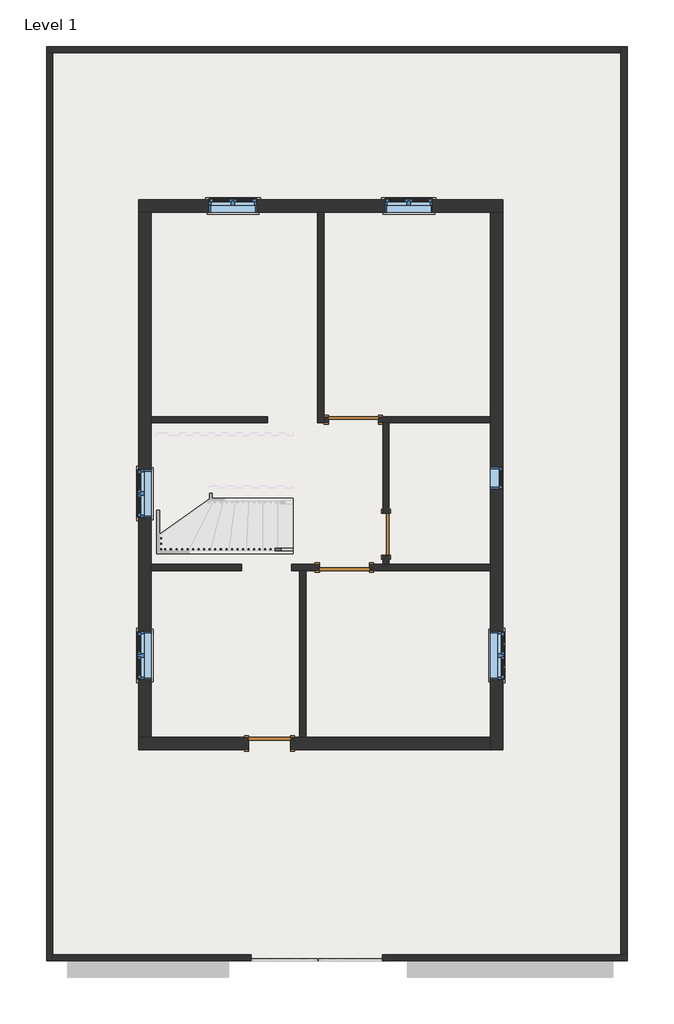
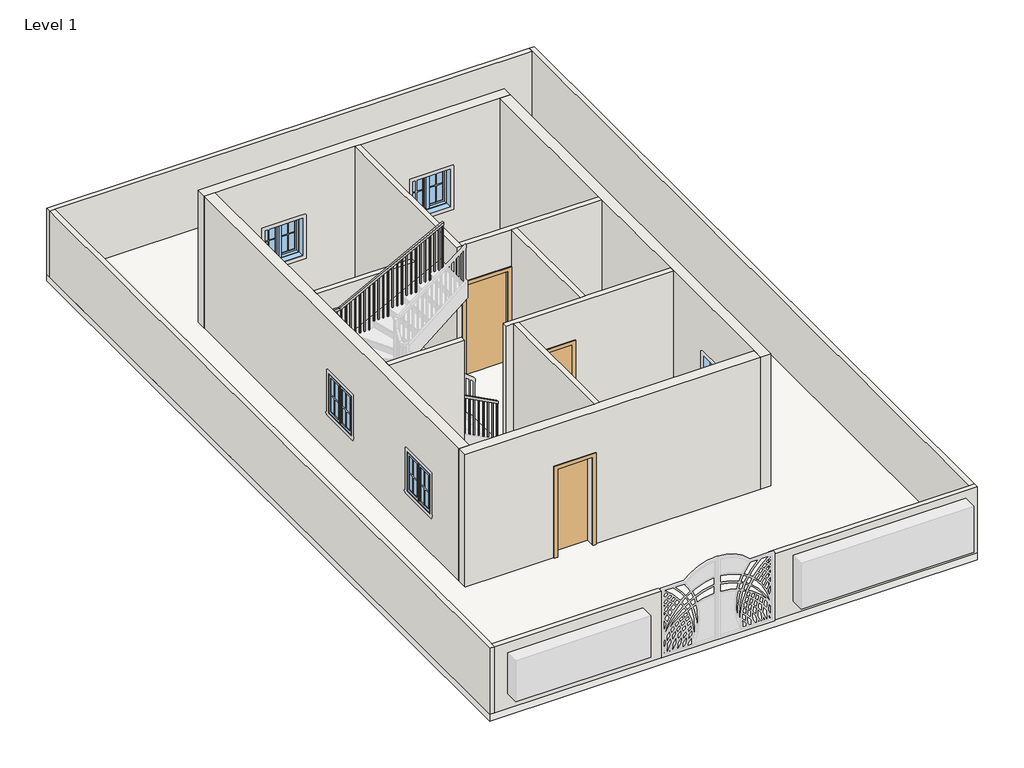
# One storey, part 1 of 2: 16 walls, 6 windows, 4 doors, 1 railing, 1 slab.
"""IFC4 building model written with IfcOpenShell, lengths in millimetres."""

from ifc_helpers import new_model, si_unit, frame, origin, origin_with_axes, place, context, project, spatial, polyline, outline, extrude, faceted_brep, transform, mapped, element, save
from components import door_d8f5dbb5, door_85036156, door_305aa2a5, door_e5f9f3c4, window_aa618e30, window_339605e1

model = new_model("IFC4")

# Units and contexts
model_context = context("Model", 3, world=origin())
ifc_project = project(units=[si_unit("LENGTHUNIT", "METRE", prefix="MILLI")], contexts=[model_context])

# Site, building, storey
site = spatial("IfcSite", under=ifc_project)
building = spatial("IfcBuilding", under=site)
storey = spatial("IfcBuildingStorey", under=building, Name="Level 1", Elevation=0.0)

# Doors
placement = place(None, origin())
door_shape = door_d8f5dbb5(model_context)
element("IfcDoor", 1, ObjectType="Single-Flush : 30\" x 80\"", at=placement, inside=storey, context=model_context, shape_type="MappedRepresentation", body=[
    mapped(door_shape, transform((-82.2715692, -955.3070853, 0.0), x_axis=(0.0, -1.0, 0.0), y_axis=(1.0, 0.0, 0.0), z_axis=(0.0, 0.0, 1.0))),
])
door_2_shape = door_85036156(model_context)
element("IfcDoor", 2, ObjectType="Single-Flush : 30\" x 80\"", at=placement, inside=storey, context=model_context, shape_type="MappedRepresentation", body=[
    mapped(door_2_shape, transform((-2212.5949167, -4784.3570853, 0.0), x_axis=(-1.0, 0.0, 0.0), y_axis=(0.0, -1.0, 0.0), z_axis=(0.0, 0.0, 1.0))),
])
door_3_shape = door_305aa2a5(model_context)
element("IfcDoor", 3, ObjectType="Single-Flush : 36\" x 84\"", at=placement, inside=storey, context=model_context, shape_type="MappedRepresentation", body=[
    mapped(door_3_shape, transform((-677.5332429, 1140.1929147, 0.0), x_axis=(-1.0, 0.0, 0.0), y_axis=(0.0, -1.0, 0.0), z_axis=(0.0, 0.0, 1.0))),
])
door_4_shape = door_e5f9f3c4(model_context)
element("IfcDoor", 4, ObjectType="Single-Flush : 36\" x 84\"", at=placement, inside=storey, context=model_context, shape_type="MappedRepresentation", body=[
    mapped(door_4_shape, transform((-842.6332429, -1564.9070853, 0.0), x_axis=(-1.0, 0.0, 0.0), y_axis=(0.0, -1.0, 0.0), z_axis=(0.0, 0.0, 1.0))),
])

# Railing
element("IfcRailing", 5, ObjectType="Handrail - Rectangular", at=placement, inside=storey, context=model_context, shape_type="SolidModel", body=[
    faceted_brep([(-1783.4132248, -1260.1070853, 1083.7333333), (-1783.4132248, -1260.1070853, 1026.2742652), (-1783.4132248, -1209.3070853, 1026.2742652), (-1783.4132248, -1209.3070853, 1083.7333333), (-4041.1382869, -1260.1070853, 2277.0239201), (-4053.7373514, -1260.1070853, 2226.2239201), (-4053.7373514, -1209.3070853, 2226.2239201), (-4041.1382869, -1209.3070853, 2277.0239201), (-4225.5449167, -1260.1070853, 2277.0239201), (-4225.5449167, -1260.1070853, 2226.2239201), (-4174.7449167, -1209.3070853, 2226.2239201), (-4174.7449167, -1209.3070853, 2277.0239201), (-4225.5449167, -972.7952032, 2277.0239201), (-4225.5449167, -964.8446271, 2226.2239201), (-4174.7449167, -964.8446271, 2226.2239201), (-4174.7449167, -972.7952032, 2277.0239201), (-4225.5449167, 560.7810325, 2769.1094132), (-4225.5449167, 568.7316087, 2718.3094132), (-4174.7449167, 568.7316087, 2718.3094132), (-4174.7449167, 560.7810325, 2769.1094132), (-4225.5449167, 848.0929147, 2769.1094132), (-4225.5449167, 848.0929147, 2718.3094132), (-4174.7449167, 797.2929147, 2718.3094132), (-4174.7449167, 797.2929147, 2769.1094132), (-4041.1382869, 848.0929147, 2769.1094132), (-4028.5392223, 848.0929147, 2718.3094132), (-4028.5392223, 797.2929147, 2718.3094132), (-4041.1382869, 797.2929147, 2769.1094132), (-1783.4132248, 848.0929147, 3962.4), (-1783.4132248, 797.2929147, 3962.4), (-1783.4132248, 797.2929147, 3904.9409318), (-1783.4132248, 848.0929147, 3904.9409318)], [[[0, 1, 2, 3]], [[1, 0, 4, 5]], [[2, 1, 5, 6]], [[3, 2, 6, 7]], [[0, 3, 7, 4]], [[5, 4, 8, 9]], [[6, 5, 9, 10]], [[7, 6, 10, 11]], [[4, 7, 11, 8]], [[9, 8, 12, 13]], [[10, 9, 13, 14]], [[11, 10, 14, 15]], [[8, 11, 15, 12]], [[13, 12, 16, 17]], [[14, 13, 17, 18]], [[15, 14, 18, 19]], [[12, 15, 19, 16]], [[17, 16, 20, 21]], [[18, 17, 21, 22]], [[19, 18, 22, 23]], [[16, 19, 23, 20]], [[21, 20, 24, 25]], [[22, 21, 25, 26]], [[23, 22, 26, 27]], [[20, 23, 27, 24]], [[28, 29, 30, 31]], [[25, 24, 28, 31]], [[26, 25, 31, 30]], [[27, 26, 30, 29]], [[24, 27, 29, 28]]]),
    extrude(outline(polyline([(3857.6597858, -1872.8699167), (2878.6666667, -1872.8699167), (2878.6666667, -1853.8199167), (3867.7284102, -1853.8199167), (3857.6597858, -1872.8699167)])), frame((0.0, 813.1679147, 0.0), z_axis=(0.0, 1.0, 0.0), x_axis=(0.0, 0.0, 1.0)), (0.0, 0.0, 1.0), 19.05),
    extrude(outline(polyline([(3803.9604556, -1974.4699167), (2878.6666667, -1974.4699167), (2878.6666667, -1955.4199167), (3814.02908, -1955.4199167), (3803.9604556, -1974.4699167)])), frame((0.0, 813.1679147, 0.0), z_axis=(0.0, 1.0, 0.0), x_axis=(0.0, 0.0, 1.0)), (0.0, 0.0, 1.0), 19.05),
    extrude(outline(polyline([(3750.2611254, -2076.0699167), (2709.3333333, -2076.0699167), (2709.3333333, -2057.0199167), (3760.3297498, -2057.0199167), (3750.2611254, -2076.0699167)])), frame((0.0, 813.1679147, 0.0), z_axis=(0.0, 1.0, 0.0), x_axis=(0.0, 0.0, 1.0)), (0.0, 0.0, 1.0), 19.05),
    extrude(outline(polyline([(3696.5617952, -2177.6699167), (2709.3333333, -2177.6699167), (2709.3333333, -2158.6199167), (3706.6304196, -2158.6199167), (3696.5617952, -2177.6699167)])), frame((0.0, 813.1679147, 0.0), z_axis=(0.0, 1.0, 0.0), x_axis=(0.0, 0.0, 1.0)), (0.0, 0.0, 1.0), 19.05),
    extrude(outline(polyline([(3642.862465, -2279.2699167), (2709.3333333, -2279.2699167), (2709.3333333, -2260.2199167), (3652.9310894, -2260.2199167), (3642.862465, -2279.2699167)])), frame((0.0, 813.1679147, 0.0), z_axis=(0.0, 1.0, 0.0), x_axis=(0.0, 0.0, 1.0)), (0.0, 0.0, 1.0), 19.05),
    extrude(outline(polyline([(3589.1631348, -2380.8699167), (2540.0, -2380.8699167), (2540.0, -2361.8199167), (3599.2317592, -2361.8199167), (3589.1631348, -2380.8699167)])), frame((0.0, 813.1679147, 0.0), z_axis=(0.0, 1.0, 0.0), x_axis=(0.0, 0.0, 1.0)), (0.0, 0.0, 1.0), 19.05),
    extrude(outline(polyline([(3535.4638046, -2482.4699167), (2540.0, -2482.4699167), (2540.0, -2463.4199167), (3545.532429, -2463.4199167), (3535.4638046, -2482.4699167)])), frame((0.0, 813.1679147, 0.0), z_axis=(0.0, 1.0, 0.0), x_axis=(0.0, 0.0, 1.0)), (0.0, 0.0, 1.0), 19.05),
    extrude(outline(polyline([(3481.7644744, -2584.0699167), (2540.0, -2584.0699167), (2540.0, -2565.0199167), (3491.8330988, -2565.0199167), (3481.7644744, -2584.0699167)])), frame((0.0, 813.1679147, 0.0), z_axis=(0.0, 1.0, 0.0), x_axis=(0.0, 0.0, 1.0)), (0.0, 0.0, 1.0), 19.05),
    extrude(outline(polyline([(3428.0651442, -2685.6699167), (2370.6666667, -2685.6699167), (2370.6666667, -2666.6199167), (3438.1337686, -2666.6199167), (3428.0651442, -2685.6699167)])), frame((0.0, 813.1679147, 0.0), z_axis=(0.0, 1.0, 0.0), x_axis=(0.0, 0.0, 1.0)), (0.0, 0.0, 1.0), 19.05),
    extrude(outline(polyline([(3374.365814, -2787.2699167), (2370.6666667, -2787.2699167), (2370.6666667, -2768.2199167), (3384.4344384, -2768.2199167), (3374.365814, -2787.2699167)])), frame((0.0, 813.1679147, 0.0), z_axis=(0.0, 1.0, 0.0), x_axis=(0.0, 0.0, 1.0)), (0.0, 0.0, 1.0), 19.05),
    extrude(outline(polyline([(3320.6664838, -2888.8699167), (2370.6666667, -2888.8699167), (2370.6666667, -2869.8199167), (3330.7351082, -2869.8199167), (3320.6664838, -2888.8699167)])), frame((0.0, 813.1679147, 0.0), z_axis=(0.0, 1.0, 0.0), x_axis=(0.0, 0.0, 1.0)), (0.0, 0.0, 1.0), 19.05),
    extrude(outline(polyline([(3266.9671536, -2990.4699167), (2201.3333333, -2990.4699167), (2201.3333333, -2971.4199167), (3277.035778, -2971.4199167), (3266.9671536, -2990.4699167)])), frame((0.0, 813.1679147, 0.0), z_axis=(0.0, 1.0, 0.0), x_axis=(0.0, 0.0, 1.0)), (0.0, 0.0, 1.0), 19.05),
    extrude(outline(polyline([(3213.2678234, -3092.0699167), (2201.3333333, -3092.0699167), (2201.3333333, -3073.0199167), (3223.3364478, -3073.0199167), (3213.2678234, -3092.0699167)])), frame((0.0, 813.1679147, 0.0), z_axis=(0.0, 1.0, 0.0), x_axis=(0.0, 0.0, 1.0)), (0.0, 0.0, 1.0), 19.05),
    extrude(outline(polyline([(3159.5684932, -3193.6699167), (2201.3333333, -3193.6699167), (2201.3333333, -3174.6199167), (3169.6371176, -3174.6199167), (3159.5684932, -3193.6699167)])), frame((0.0, 813.1679147, 0.0), z_axis=(0.0, 1.0, 0.0), x_axis=(0.0, 0.0, 1.0)), (0.0, 0.0, 1.0), 19.05),
    extrude(outline(polyline([(3105.869163, -3295.2699167), (2201.3333333, -3295.2699167), (2201.3333333, -3276.2199167), (3115.9377874, -3276.2199167), (3105.869163, -3295.2699167)])), frame((0.0, 813.1679147, 0.0), z_axis=(0.0, 1.0, 0.0), x_axis=(0.0, 0.0, 1.0)), (0.0, 0.0, 1.0), 19.05),
    extrude(outline(polyline([(3052.1698328, -3396.8699167), (2032.0, -3396.8699167), (2032.0, -3377.8199167), (3062.2384572, -3377.8199167), (3052.1698328, -3396.8699167)])), frame((0.0, 813.1679147, 0.0), z_axis=(0.0, 1.0, 0.0), x_axis=(0.0, 0.0, 1.0)), (0.0, 0.0, 1.0), 19.05),
    extrude(outline(polyline([(2998.4705026, -3498.4699167), (2032.0, -3498.4699167), (2032.0, -3479.4199167), (3008.539127, -3479.4199167), (2998.4705026, -3498.4699167)])), frame((0.0, 813.1679147, 0.0), z_axis=(0.0, 1.0, 0.0), x_axis=(0.0, 0.0, 1.0)), (0.0, 0.0, 1.0), 19.05),
    extrude(outline(polyline([(2944.7711724, -3600.0699167), (2032.0, -3600.0699167), (2032.0, -3581.0199167), (2954.8397968, -3581.0199167), (2944.7711724, -3600.0699167)])), frame((0.0, 813.1679147, 0.0), z_axis=(0.0, 1.0, 0.0), x_axis=(0.0, 0.0, 1.0)), (0.0, 0.0, 1.0), 19.05),
    extrude(outline(polyline([(2891.0718422, -3701.6699167), (2032.0, -3701.6699167), (2032.0, -3682.6199167), (2901.1404666, -3682.6199167), (2891.0718422, -3701.6699167)])), frame((0.0, 813.1679147, 0.0), z_axis=(0.0, 1.0, 0.0), x_axis=(0.0, 0.0, 1.0)), (0.0, 0.0, 1.0), 19.05),
    extrude(outline(polyline([(2837.372512, -3803.2699167), (1862.6666667, -3803.2699167), (1862.6666667, -3784.2199167), (2847.4411364, -3784.2199167), (2837.372512, -3803.2699167)])), frame((0.0, 813.1679147, 0.0), z_axis=(0.0, 1.0, 0.0), x_axis=(0.0, 0.0, 1.0)), (0.0, 0.0, 1.0), 19.05),
    extrude(outline(polyline([(2783.6731818, -3904.8699167), (1862.6666667, -3904.8699167), (1862.6666667, -3885.8199167), (2793.7418062, -3885.8199167), (2783.6731818, -3904.8699167)])), frame((0.0, 813.1679147, 0.0), z_axis=(0.0, 1.0, 0.0), x_axis=(0.0, 0.0, 1.0)), (0.0, 0.0, 1.0), 19.05),
    extrude(outline(polyline([(2729.9738516, -4006.4699167), (1862.6666667, -4006.4699167), (1862.6666667, -3987.4199167), (2740.042476, -3987.4199167), (2729.9738516, -4006.4699167)])), frame((0.0, 813.1679147, 0.0), z_axis=(0.0, 1.0, 0.0), x_axis=(0.0, 0.0, 1.0)), (0.0, 0.0, 1.0), 19.05),
    extrude(outline(polyline([(-4108.0699167, 832.2179147), (-4089.0199167, 832.2179147), (-4089.0199167, 813.1679147), (-4108.0699167, 813.1679147), (-4108.0699167, 832.2179147)])), frame((0.0, 0.0, 1862.6666667), z_axis=(0.0, 0.0, 1.0), x_axis=(1.0, 0.0, 0.0)), (0.0, 0.0, 1.0), 855.6427466),
    extrude(outline(polyline([(-4209.6699167, 787.7679147), (-4209.6699167, 806.8179147), (-4190.6199167, 806.8179147), (-4190.6199167, 787.7679147), (-4209.6699167, 787.7679147)])), frame((0.0, 0.0, 1862.6666667), z_axis=(0.0, 0.0, 1.0), x_axis=(1.0, 0.0, 0.0)), (0.0, 0.0, 1.0), 855.6427466),
    extrude(outline(polyline([(-4209.6699167, 686.1679147), (-4209.6699167, 705.2179147), (-4190.6199167, 705.2179147), (-4190.6199167, 686.1679147), (-4209.6699167, 686.1679147)])), frame((0.0, 0.0, 1862.6666667), z_axis=(0.0, 0.0, 1.0), x_axis=(1.0, 0.0, 0.0)), (0.0, 0.0, 1.0), 855.6427466),
    extrude(outline(polyline([(-4209.6699167, 584.5679147), (-4209.6699167, 603.6179147), (-4190.6199167, 603.6179147), (-4190.6199167, 584.5679147), (-4209.6699167, 584.5679147)])), frame((0.0, 0.0, 1862.6666667), z_axis=(0.0, 0.0, 1.0), x_axis=(1.0, 0.0, 0.0)), (0.0, 0.0, 1.0), 855.6427466),
    extrude(outline(polyline([(502.0179147, 2696.9026907), (502.0179147, 1693.3333333), (482.9679147, 1693.3333333), (482.9679147, 2690.7900316), (502.0179147, 2696.9026907)])), frame((-4209.6699167, 0.0, 0.0), z_axis=(1.0, 0.0, 0.0), x_axis=(0.0, 1.0, 0.0)), (0.0, 0.0, 1.0), 19.05),
    extrude(outline(polyline([(400.4179147, 2664.3018425), (400.4179147, 1693.3333333), (381.3679147, 1693.3333333), (381.3679147, 2658.1891834), (400.4179147, 2664.3018425)])), frame((-4209.6699167, 0.0, 0.0), z_axis=(1.0, 0.0, 0.0), x_axis=(0.0, 1.0, 0.0)), (0.0, 0.0, 1.0), 19.05),
    extrude(outline(polyline([(298.8179147, 2631.7009942), (298.8179147, 1693.3333333), (279.7679147, 1693.3333333), (279.7679147, 2625.5883352), (298.8179147, 2631.7009942)])), frame((-4209.6699167, 0.0, 0.0), z_axis=(1.0, 0.0, 0.0), x_axis=(0.0, 1.0, 0.0)), (0.0, 0.0, 1.0), 19.05),
    extrude(outline(polyline([(197.2179147, 2599.100146), (197.2179147, 1693.3333333), (178.1679147, 1693.3333333), (178.1679147, 2592.987487), (197.2179147, 2599.100146)])), frame((-4209.6699167, 0.0, 0.0), z_axis=(1.0, 0.0, 0.0), x_axis=(0.0, 1.0, 0.0)), (0.0, 0.0, 1.0), 19.05),
    extrude(outline(polyline([(95.6179147, 2566.4992978), (95.6179147, 1693.3333333), (76.5679147, 1693.3333333), (76.5679147, 2560.3866387), (95.6179147, 2566.4992978)])), frame((-4209.6699167, 0.0, 0.0), z_axis=(1.0, 0.0, 0.0), x_axis=(0.0, 1.0, 0.0)), (0.0, 0.0, 1.0), 19.05),
    extrude(outline(polyline([(-5.9820853, 2533.8984495), (-5.9820853, 1524.0), (-25.0320853, 1524.0), (-25.0320853, 2527.7857905), (-5.9820853, 2533.8984495)])), frame((-4209.6699167, 0.0, 0.0), z_axis=(1.0, 0.0, 0.0), x_axis=(0.0, 1.0, 0.0)), (0.0, 0.0, 1.0), 19.05),
    extrude(outline(polyline([(-107.5820853, 2501.2976013), (-107.5820853, 1524.0), (-126.6320853, 1524.0), (-126.6320853, 2495.1849423), (-107.5820853, 2501.2976013)])), frame((-4209.6699167, 0.0, 0.0), z_axis=(1.0, 0.0, 0.0), x_axis=(0.0, 1.0, 0.0)), (0.0, 0.0, 1.0), 19.05),
    extrude(outline(polyline([(-209.1820853, 2468.6967531), (-209.1820853, 1524.0), (-228.2320853, 1524.0), (-228.2320853, 2462.5840941), (-209.1820853, 2468.6967531)])), frame((-4209.6699167, 0.0, 0.0), z_axis=(1.0, 0.0, 0.0), x_axis=(0.0, 1.0, 0.0)), (0.0, 0.0, 1.0), 19.05),
    extrude(outline(polyline([(-310.7820853, 2436.0959049), (-310.7820853, 1524.0), (-329.8320853, 1524.0), (-329.8320853, 2429.9832458), (-310.7820853, 2436.0959049)])), frame((-4209.6699167, 0.0, 0.0), z_axis=(1.0, 0.0, 0.0), x_axis=(0.0, 1.0, 0.0)), (0.0, 0.0, 1.0), 19.05),
    extrude(outline(polyline([(-412.3820853, 2403.4950566), (-412.3820853, 1524.0), (-431.4320853, 1524.0), (-431.4320853, 2397.3823976), (-412.3820853, 2403.4950566)])), frame((-4209.6699167, 0.0, 0.0), z_axis=(1.0, 0.0, 0.0), x_axis=(0.0, 1.0, 0.0)), (0.0, 0.0, 1.0), 19.05),
    extrude(outline(polyline([(-513.9820853, 2370.8942084), (-513.9820853, 1354.6666667), (-533.0320853, 1354.6666667), (-533.0320853, 2364.7815494), (-513.9820853, 2370.8942084)])), frame((-4209.6699167, 0.0, 0.0), z_axis=(1.0, 0.0, 0.0), x_axis=(0.0, 1.0, 0.0)), (0.0, 0.0, 1.0), 19.05),
    extrude(outline(polyline([(-615.5820853, 2338.2933602), (-615.5820853, 1354.6666667), (-634.6320853, 1354.6666667), (-634.6320853, 2332.1807011), (-615.5820853, 2338.2933602)])), frame((-4209.6699167, 0.0, 0.0), z_axis=(1.0, 0.0, 0.0), x_axis=(0.0, 1.0, 0.0)), (0.0, 0.0, 1.0), 19.05),
    extrude(outline(polyline([(-717.1820853, 2305.692512), (-717.1820853, 1354.6666667), (-736.2320853, 1354.6666667), (-736.2320853, 2299.5798529), (-717.1820853, 2305.692512)])), frame((-4209.6699167, 0.0, 0.0), z_axis=(1.0, 0.0, 0.0), x_axis=(0.0, 1.0, 0.0)), (0.0, 0.0, 1.0), 19.05),
    extrude(outline(polyline([(-818.7820853, 2273.0916637), (-818.7820853, 1354.6666667), (-837.8320853, 1354.6666667), (-837.8320853, 2266.9790047), (-818.7820853, 2273.0916637)])), frame((-4209.6699167, 0.0, 0.0), z_axis=(1.0, 0.0, 0.0), x_axis=(0.0, 1.0, 0.0)), (0.0, 0.0, 1.0), 19.05),
    extrude(outline(polyline([(-920.3820853, 2240.4908155), (-920.3820853, 1354.6666667), (-939.4320853, 1354.6666667), (-939.4320853, 2234.3781565), (-920.3820853, 2240.4908155)])), frame((-4209.6699167, 0.0, 0.0), z_axis=(1.0, 0.0, 0.0), x_axis=(0.0, 1.0, 0.0)), (0.0, 0.0, 1.0), 19.05),
    extrude(outline(polyline([(-4209.6699167, -1041.0320853), (-4209.6699167, -1021.9820853), (-4190.6199167, -1021.9820853), (-4190.6199167, -1041.0320853), (-4209.6699167, -1041.0320853)])), frame((0.0, 0.0, 1185.3333333), z_axis=(0.0, 0.0, 1.0), x_axis=(1.0, 0.0, 0.0)), (0.0, 0.0, 1.0), 1040.8905868),
    extrude(outline(polyline([(-4209.6699167, -1142.6320853), (-4209.6699167, -1123.5820853), (-4190.6199167, -1123.5820853), (-4190.6199167, -1142.6320853), (-4209.6699167, -1142.6320853)])), frame((0.0, 0.0, 1185.3333333), z_axis=(0.0, 0.0, 1.0), x_axis=(1.0, 0.0, 0.0)), (0.0, 0.0, 1.0), 1040.8905868),
    extrude(outline(polyline([(-4110.6882248, -1244.2320853), (-4129.7382248, -1244.2320853), (-4129.7382248, -1225.1820853), (-4110.6882248, -1225.1820853), (-4110.6882248, -1244.2320853)])), frame((0.0, 0.0, 1185.3333333), z_axis=(0.0, 0.0, 1.0), x_axis=(1.0, 0.0, 0.0)), (0.0, 0.0, 1.0), 1040.8905868),
    extrude(outline(polyline([(2212.6938418, -4028.1382248), (1185.3333333, -4028.1382248), (1185.3333333, -4009.0882248), (2202.6252174, -4009.0882248), (2212.6938418, -4028.1382248)])), frame((0.0, -1244.2320853, 0.0), z_axis=(0.0, 1.0, 0.0), x_axis=(0.0, 0.0, 1.0)), (0.0, 0.0, 1.0), 19.05),
    extrude(outline(polyline([(2158.9945116, -3926.5382248), (1185.3333333, -3926.5382248), (1185.3333333, -3907.4882248), (2148.9258872, -3907.4882248), (2158.9945116, -3926.5382248)])), frame((0.0, -1244.2320853, 0.0), z_axis=(0.0, 1.0, 0.0), x_axis=(0.0, 0.0, 1.0)), (0.0, 0.0, 1.0), 19.05),
    extrude(outline(polyline([(2105.2951814, -3824.9382248), (1185.3333333, -3824.9382248), (1185.3333333, -3805.8882248), (2095.226557, -3805.8882248), (2105.2951814, -3824.9382248)])), frame((0.0, -1244.2320853, 0.0), z_axis=(0.0, 1.0, 0.0), x_axis=(0.0, 0.0, 1.0)), (0.0, 0.0, 1.0), 19.05),
    extrude(outline(polyline([(2051.5958512, -3723.3382248), (1185.3333333, -3723.3382248), (1185.3333333, -3704.2882248), (2041.5272268, -3704.2882248), (2051.5958512, -3723.3382248)])), frame((0.0, -1244.2320853, 0.0), z_axis=(0.0, 1.0, 0.0), x_axis=(0.0, 0.0, 1.0)), (0.0, 0.0, 1.0), 19.05),
    extrude(outline(polyline([(1997.896521, -3621.7382248), (1016.0, -3621.7382248), (1016.0, -3602.6882248), (1987.8278966, -3602.6882248), (1997.896521, -3621.7382248)])), frame((0.0, -1244.2320853, 0.0), z_axis=(0.0, 1.0, 0.0), x_axis=(0.0, 0.0, 1.0)), (0.0, 0.0, 1.0), 19.05),
    extrude(outline(polyline([(1944.1971908, -3520.1382248), (1016.0, -3520.1382248), (1016.0, -3501.0882248), (1934.1285664, -3501.0882248), (1944.1971908, -3520.1382248)])), frame((0.0, -1244.2320853, 0.0), z_axis=(0.0, 1.0, 0.0), x_axis=(0.0, 0.0, 1.0)), (0.0, 0.0, 1.0), 19.05),
    extrude(outline(polyline([(1890.4978606, -3418.5382248), (1016.0, -3418.5382248), (1016.0, -3399.4882248), (1880.4292362, -3399.4882248), (1890.4978606, -3418.5382248)])), frame((0.0, -1244.2320853, 0.0), z_axis=(0.0, 1.0, 0.0), x_axis=(0.0, 0.0, 1.0)), (0.0, 0.0, 1.0), 19.05),
    extrude(outline(polyline([(1836.7985304, -3316.9382248), (1016.0, -3316.9382248), (1016.0, -3297.8882248), (1826.729906, -3297.8882248), (1836.7985304, -3316.9382248)])), frame((0.0, -1244.2320853, 0.0), z_axis=(0.0, 1.0, 0.0), x_axis=(0.0, 0.0, 1.0)), (0.0, 0.0, 1.0), 19.05),
    extrude(outline(polyline([(1783.0992002, -3215.3382248), (846.6666667, -3215.3382248), (846.6666667, -3196.2882248), (1773.0305758, -3196.2882248), (1783.0992002, -3215.3382248)])), frame((0.0, -1244.2320853, 0.0), z_axis=(0.0, 1.0, 0.0), x_axis=(0.0, 0.0, 1.0)), (0.0, 0.0, 1.0), 19.05),
    extrude(outline(polyline([(1729.39987, -3113.7382248), (846.6666667, -3113.7382248), (846.6666667, -3094.6882248), (1719.3312456, -3094.6882248), (1729.39987, -3113.7382248)])), frame((0.0, -1244.2320853, 0.0), z_axis=(0.0, 1.0, 0.0), x_axis=(0.0, 0.0, 1.0)), (0.0, 0.0, 1.0), 19.05),
    extrude(outline(polyline([(1675.7005398, -3012.1382248), (846.6666667, -3012.1382248), (846.6666667, -2993.0882248), (1665.6319154, -2993.0882248), (1675.7005398, -3012.1382248)])), frame((0.0, -1244.2320853, 0.0), z_axis=(0.0, 1.0, 0.0), x_axis=(0.0, 0.0, 1.0)), (0.0, 0.0, 1.0), 19.05),
    extrude(outline(polyline([(1622.0012096, -2910.5382248), (677.3333333, -2910.5382248), (677.3333333, -2891.4882248), (1611.9325852, -2891.4882248), (1622.0012096, -2910.5382248)])), frame((0.0, -1244.2320853, 0.0), z_axis=(0.0, 1.0, 0.0), x_axis=(0.0, 0.0, 1.0)), (0.0, 0.0, 1.0), 19.05),
    extrude(outline(polyline([(1568.3018794, -2808.9382248), (677.3333333, -2808.9382248), (677.3333333, -2789.8882248), (1558.233255, -2789.8882248), (1568.3018794, -2808.9382248)])), frame((0.0, -1244.2320853, 0.0), z_axis=(0.0, 1.0, 0.0), x_axis=(0.0, 0.0, 1.0)), (0.0, 0.0, 1.0), 19.05),
    extrude(outline(polyline([(1514.6025492, -2707.3382248), (677.3333333, -2707.3382248), (677.3333333, -2688.2882248), (1504.5339248, -2688.2882248), (1514.6025492, -2707.3382248)])), frame((0.0, -1244.2320853, 0.0), z_axis=(0.0, 1.0, 0.0), x_axis=(0.0, 0.0, 1.0)), (0.0, 0.0, 1.0), 19.05),
    extrude(outline(polyline([(1460.903219, -2605.7382248), (508.0, -2605.7382248), (508.0, -2586.6882248), (1450.8345946, -2586.6882248), (1460.903219, -2605.7382248)])), frame((0.0, -1244.2320853, 0.0), z_axis=(0.0, 1.0, 0.0), x_axis=(0.0, 0.0, 1.0)), (0.0, 0.0, 1.0), 19.05),
    extrude(outline(polyline([(1407.2038888, -2504.1382248), (508.0, -2504.1382248), (508.0, -2485.0882248), (1397.1352644, -2485.0882248), (1407.2038888, -2504.1382248)])), frame((0.0, -1244.2320853, 0.0), z_axis=(0.0, 1.0, 0.0), x_axis=(0.0, 0.0, 1.0)), (0.0, 0.0, 1.0), 19.05),
    extrude(outline(polyline([(1353.5045586, -2402.5382248), (508.0, -2402.5382248), (508.0, -2383.4882248), (1343.4359342, -2383.4882248), (1353.5045586, -2402.5382248)])), frame((0.0, -1244.2320853, 0.0), z_axis=(0.0, 1.0, 0.0), x_axis=(0.0, 0.0, 1.0)), (0.0, 0.0, 1.0), 19.05),
    extrude(outline(polyline([(1299.8052284, -2300.9382248), (338.6666667, -2300.9382248), (338.6666667, -2281.8882248), (1289.736604, -2281.8882248), (1299.8052284, -2300.9382248)])), frame((0.0, -1244.2320853, 0.0), z_axis=(0.0, 1.0, 0.0), x_axis=(0.0, 0.0, 1.0)), (0.0, 0.0, 1.0), 19.05),
    extrude(outline(polyline([(1246.1058982, -2199.3382248), (338.6666667, -2199.3382248), (338.6666667, -2180.2882248), (1236.0372738, -2180.2882248), (1246.1058982, -2199.3382248)])), frame((0.0, -1244.2320853, 0.0), z_axis=(0.0, 1.0, 0.0), x_axis=(0.0, 0.0, 1.0)), (0.0, 0.0, 1.0), 19.05),
    extrude(outline(polyline([(1192.406568, -2097.7382248), (338.6666667, -2097.7382248), (338.6666667, -2078.6882248), (1182.3379436, -2078.6882248), (1192.406568, -2097.7382248)])), frame((0.0, -1244.2320853, 0.0), z_axis=(0.0, 1.0, 0.0), x_axis=(0.0, 0.0, 1.0)), (0.0, 0.0, 1.0), 19.05),
    extrude(outline(polyline([(1138.7072378, -1996.1382248), (169.3333333, -1996.1382248), (169.3333333, -1977.0882248), (1128.6386134, -1977.0882248), (1138.7072378, -1996.1382248)])), frame((0.0, -1244.2320853, 0.0), z_axis=(0.0, 1.0, 0.0), x_axis=(0.0, 0.0, 1.0)), (0.0, 0.0, 1.0), 19.05),
    extrude(outline(polyline([(1085.0079076, -1894.5382248), (169.3333333, -1894.5382248), (169.3333333, -1875.4882248), (1074.9392831, -1875.4882248), (1085.0079076, -1894.5382248)])), frame((0.0, -1244.2320853, 0.0), z_axis=(0.0, 1.0, 0.0), x_axis=(0.0, 0.0, 1.0)), (0.0, 0.0, 1.0), 19.05),
    extrude(outline(polyline([(-4209.6699167, 813.1679147), (-4209.6699167, 832.2179147), (-4190.6199167, 832.2179147), (-4190.6199167, 813.1679147), (-4209.6699167, 813.1679147)])), frame((0.0, 0.0, 1862.6666667), z_axis=(0.0, 0.0, 1.0), x_axis=(1.0, 0.0, 0.0)), (0.0, 0.0, 1.0), 855.6427466),
    extrude(outline(polyline([(-4190.6199167, -1244.2320853), (-4209.6699167, -1244.2320853), (-4209.6699167, -1225.1820853), (-4190.6199167, -1225.1820853), (-4190.6199167, -1244.2320853)])), frame((0.0, 0.0, 1185.3333333), z_axis=(0.0, 0.0, 1.0), x_axis=(1.0, 0.0, 0.0)), (0.0, 0.0, 1.0), 1040.8905868),
    extrude(outline(polyline([(3894.8723074, -1802.4632248), (2878.6666667, -1802.4632248), (2878.6666667, -1783.4132248), (3904.9409318, -1783.4132248), (3894.8723074, -1802.4632248)])), frame((0.0, 813.1679147, 0.0), z_axis=(0.0, 1.0, 0.0), x_axis=(0.0, 0.0, 1.0)), (0.0, 0.0, 1.0), 19.05),
    extrude(outline(polyline([(1036.3428896, -1802.4632248), (169.3333333, -1802.4632248), (169.3333333, -1783.4132248), (1026.2742652, -1783.4132248), (1036.3428896, -1802.4632248)])), frame((0.0, -1244.2320853, 0.0), z_axis=(0.0, 1.0, 0.0), x_axis=(0.0, 0.0, 1.0)), (0.0, 0.0, 1.0), 19.05),
])

# Slab
element("IfcSlab", 6, ObjectType="Generic - 12\"", at=placement, inside=storey, context=model_context, shape_type="SweptSolid", body=[
    extrude(outline(polyline([(4334.3546213, 7965.8324364), (4334.3546213, -8760.0675636), (-6295.5453787, -8760.0675636), (-6295.5453787, 7965.8324364), (4334.3546213, 7965.8324364)])), frame((0.0, 0.0, -152.4), z_axis=(0.0, 0.0, 1.0), x_axis=(1.0, 0.0, 0.0)), (0.0, 0.0, 1.0), 152.4),
])

# Walls
element("IfcWall", 7, ObjectType="WALL4.5\"", at=placement, inside=storey, context=model_context, shape_type="Brep", body=[
    faceted_brep([(-1329.9449167, 4931.1429147, 0.0), (-1329.9449167, 1083.0429147, 0.0), (-1329.9449167, 1083.0429147, 3048.0), (-1329.9449167, 4931.1429147, 3048.0), (-1215.6449167, 4931.1429147, 0.0), (-1215.6449167, 4931.1429147, 3048.0), (-1215.6449167, 1197.3429147, 3048.0), (-1215.6449167, 1083.0429147, 3048.0), (-1215.6449167, 1083.0429147, 0.0), (-1215.6449167, 1197.3429147, 0.0)], [[[0, 1, 2, 3]], [[4, 5, 6, 7, 8, 9]], [[1, 0, 4, 9, 8]], [[0, 3, 5, 4]], [[2, 1, 8, 7]], [[3, 2, 7, 6, 5]]]),
])
element("IfcWall", 8, ObjectType="WALL4.5\"", at=placement, inside=storey, context=model_context, shape_type="Brep", body=[
    faceted_brep([(-1215.6449167, 1083.0429147, 0.0), (-1134.7332429, 1083.0429147, 0.0), (-1134.7332429, 1083.0429147, 2133.6), (-220.3332429, 1083.0429147, 2133.6), (-220.3332429, 1083.0429147, 0.0), (-139.4215692, 1083.0429147, 0.0), (-25.1215692, 1083.0429147, 0.0), (1832.3550833, 1083.0429147, 0.0), (1832.3550833, 1083.0429147, 3048.0), (-25.1215692, 1083.0429147, 3048.0), (-139.4215692, 1083.0429147, 3048.0), (-1215.6449167, 1083.0429147, 3048.0), (-1134.7332429, 1197.3429147, 2133.6), (-1134.7332429, 1197.3429147, 0.0), (-1215.6449167, 1197.3429147, 0.0), (-1215.6449167, 1197.3429147, 3048.0), (1832.3550833, 1197.3429147, 3048.0), (1832.3550833, 1197.3429147, 0.0), (-220.3332429, 1197.3429147, 0.0), (-220.3332429, 1197.3429147, 2133.6)], [[[0, 1, 2, 3, 4, 5, 6, 7, 8, 9, 10, 11]], [[12, 13, 14, 15, 16, 17, 18, 19]], [[18, 17, 7, 6, 5, 4]], [[14, 13, 1, 0]], [[0, 11, 15, 14]], [[8, 7, 17, 16]], [[2, 1, 13, 12]], [[3, 2, 12, 19]], [[4, 3, 19, 18]], [[11, 10, 9, 8, 16, 15]]]),
])
element("IfcWall", 9, ObjectType="WALL4.5\"", at=placement, inside=storey, context=model_context, shape_type="SweptSolid", body=[
    extrude(outline(polyline([(-2244.3449167, 1083.0429147), (-4377.9449167, 1083.0429147), (-4377.9449167, 1197.3429147), (-2244.3449167, 1197.3429147), (-2244.3449167, 1083.0429147)])), origin_with_axes(), (0.0, 0.0, 1.0), 3048.0),
])
element("IfcWall", 10, ObjectType="WALL4.5\"", at=placement, inside=storey, context=model_context, shape_type="SweptSolid", body=[
    extrude(outline(polyline([(-1336.3070853, 2032.0), (-1336.3070853, 0.0), (-1507.7570853, 0.0), (-1507.7570853, 3048.0), (1083.0429147, 3048.0), (1083.0429147, 0.0), (-574.3070853, 0.0), (-574.3070853, 2032.0), (-1336.3070853, 2032.0)])), frame((-139.4215692, 0.0, 0.0), z_axis=(1.0, 0.0, 0.0), x_axis=(0.0, 1.0, 0.0)), (0.0, 0.0, 1.0), 114.3),
])
element("IfcWall", 11, ObjectType="WALL4.5\"", at=placement, inside=storey, context=model_context, shape_type="SweptSolid", body=[
    extrude(outline(polyline([(-2726.9449167, -1622.0570853), (-4377.9449167, -1622.0570853), (-4377.9449167, -1507.7570853), (-2726.9449167, -1507.7570853), (-2726.9449167, -1622.0570853)])), origin_with_axes(), (0.0, 0.0, 1.0), 3048.0),
])
element("IfcWall", 12, ObjectType="WALL4.5\"", at=placement, inside=storey, context=model_context, shape_type="Brep", body=[
    faceted_brep([(-1812.5449167, -1622.0570853, 0.0), (-1660.1449167, -1622.0570853, 0.0), (-1545.8449167, -1622.0570853, 0.0), (-1299.8332429, -1622.0570853, 0.0), (-1299.8332429, -1622.0570853, 2133.6), (-385.4332429, -1622.0570853, 2133.6), (-385.4332429, -1622.0570853, 0.0), (1832.3550833, -1622.0570853, 0.0), (1832.3550833, -1622.0570853, 3048.0), (-1545.8449167, -1622.0570853, 3048.0), (-1660.1449167, -1622.0570853, 3048.0), (-1812.5449167, -1622.0570853, 3048.0), (-1299.8332429, -1507.7570853, 2133.6), (-1299.8332429, -1507.7570853, 0.0), (-1812.5449167, -1507.7570853, 0.0), (-1812.5449167, -1507.7570853, 3048.0), (-139.4215692, -1507.7570853, 3048.0), (-25.1215692, -1507.7570853, 3048.0), (1832.3550833, -1507.7570853, 3048.0), (1832.3550833, -1507.7570853, 0.0), (-25.1215692, -1507.7570853, 0.0), (-139.4215692, -1507.7570853, 0.0), (-385.4332429, -1507.7570853, 0.0), (-385.4332429, -1507.7570853, 2133.6)], [[[0, 1, 2, 3, 4, 5, 6, 7, 8, 9, 10, 11]], [[12, 13, 14, 15, 16, 17, 18, 19, 20, 21, 22, 23]], [[14, 13, 3, 2, 1, 0]], [[22, 21, 20, 19, 7, 6]], [[0, 11, 15, 14]], [[8, 7, 19, 18]], [[4, 3, 13, 12]], [[5, 4, 12, 23]], [[6, 5, 23, 22]], [[11, 10, 9, 8, 18, 17, 16, 15]]]),
])
element("IfcWall", 13, ObjectType="WALL4.5\"", at=placement, inside=storey, context=model_context, shape_type="SweptSolid", body=[
    extrude(outline(polyline([(-1660.1449167, -4670.0570853), (-1660.1449167, -1622.0570853), (-1545.8449167, -1622.0570853), (-1545.8449167, -4670.0570853), (-1660.1449167, -4670.0570853)])), origin_with_axes(), (0.0, 0.0, 1.0), 3048.0),
])
element("IfcWall", 14, ObjectType="WALL4.5\"", at=placement, inside=storey, context=model_context, shape_type="Brep", body=[
    faceted_brep([(-6295.5453787, 7851.5324364, 0.0), (-6181.2453787, 7851.5324364, 0.0), (4220.0546213, 7851.5324364, 0.0), (4220.0546213, 7851.5324364, 1524.0), (-6181.2453787, 7851.5324364, 1524.0), (-6295.5453787, 7851.5324364, 1524.0), (-6295.5453787, 7965.8324364, 0.0), (-6295.5453787, 7965.8324364, 1524.0), (4220.0546213, 7965.8324364, 1524.0), (4220.0546213, 7965.8324364, 0.0)], [[[0, 1, 2, 3, 4, 5]], [[6, 7, 8, 9]], [[2, 1, 0, 6, 9]], [[5, 4, 3, 8, 7]], [[0, 5, 7, 6]], [[3, 2, 9, 8]]]),
])
element("IfcWall", 15, ObjectType="WALL4.5\"", at=placement, inside=storey, context=model_context, shape_type="Brep", body=[
    faceted_brep([(-6181.2453787, -8760.0675636, 0.0), (-6181.2453787, -8645.7675636, 0.0), (-6181.2453787, 7851.5324364, 0.0), (-6181.2453787, 7851.5324364, 1524.0), (-6181.2453787, -8645.7675636, 1524.0), (-6181.2453787, -8760.0675636, 1524.0), (-6295.5453787, -8760.0675636, 0.0), (-6295.5453787, -8760.0675636, 1524.0), (-6295.5453787, 7851.5324364, 1524.0), (-6295.5453787, 7851.5324364, 0.0)], [[[0, 1, 2, 3, 4, 5]], [[6, 7, 8, 9]], [[2, 1, 0, 6, 9]], [[5, 4, 3, 8, 7]], [[0, 5, 7, 6]], [[3, 2, 9, 8]]]),
])
element("IfcWall", 16, ObjectType="WALL4.5\"", at=placement, inside=storey, context=model_context, shape_type="Brep", body=[
    faceted_brep([(4334.3546213, -8645.7675636, 0.0), (4220.0546213, -8645.7675636, 0.0), (-142.3953787, -8645.7675636, 0.0), (-142.3953787, -8645.7675636, 1524.0), (4220.0546213, -8645.7675636, 1524.0), (4334.3546213, -8645.7675636, 1524.0), (4334.3546213, -8760.0675636, 0.0), (4334.3546213, -8760.0675636, 1524.0), (-142.3953787, -8760.0675636, 1524.0), (-142.3953787, -8760.0675636, 0.0)], [[[0, 1, 2, 3, 4, 5]], [[6, 7, 8, 9]], [[2, 1, 0, 6, 9]], [[3, 2, 9, 8]], [[5, 4, 3, 8, 7]], [[0, 5, 7, 6]]]),
])
element("IfcWall", 17, ObjectType="WALL4.5\"", at=placement, inside=storey, context=model_context, shape_type="Brep", body=[
    faceted_brep([(4220.0546213, 7965.8324364, 0.0), (4220.0546213, 7851.5324364, 0.0), (4220.0546213, -8645.7675636, 0.0), (4220.0546213, -8645.7675636, 1524.0), (4220.0546213, 7851.5324364, 1524.0), (4220.0546213, 7965.8324364, 1524.0), (4334.3546213, 7965.8324364, 0.0), (4334.3546213, 7965.8324364, 1524.0), (4334.3546213, -8645.7675636, 1524.0), (4334.3546213, -8645.7675636, 0.0)], [[[0, 1, 2, 3, 4, 5]], [[6, 7, 8, 9]], [[2, 1, 0, 6, 9]], [[5, 4, 3, 8, 7]], [[0, 5, 7, 6]], [[3, 2, 9, 8]]]),
])
element("IfcWall", 18, ObjectType="WALL4.5\"", at=placement, inside=storey, context=model_context, shape_type="SweptSolid", body=[
    extrude(outline(polyline([(-6181.2453787, -8645.7675636), (-2552.3199167, -8645.7675636), (-2552.3199167, -8760.0675636), (-6181.2453787, -8760.0675636), (-6181.2453787, -8645.7675636)])), origin_with_axes(), (0.0, 0.0, 1.0), 1524.0),
])
element("IfcWall", 19, ObjectType="WALL9\"", at=placement, inside=storey, context=model_context, shape_type="Brep", body=[
    faceted_brep([(-4606.5449167, 4931.1429147, 0.0), (-4377.9449167, 4931.1429147, 0.0), (-1329.9449167, 4931.1429147, 0.0), (-1215.6449167, 4931.1429147, 0.0), (1832.3550833, 4931.1429147, 0.0), (2060.9550833, 4931.1429147, 0.0), (2060.9550833, 4931.1429147, 3048.0), (1832.3550833, 4931.1429147, 3048.0), (-1215.6449167, 4931.1429147, 3048.0), (-1329.9449167, 4931.1429147, 3048.0), (-4377.9449167, 4931.1429147, 3048.0), (-4606.5449167, 4931.1429147, 3048.0), (-2450.7199167, 4931.1429147, 1828.8), (-2450.7199167, 4931.1429147, 914.4), (-3314.3199167, 4931.1429147, 914.4), (-3314.3199167, 4931.1429147, 1828.8), (768.7300833, 4931.1429147, 1828.8), (768.7300833, 4931.1429147, 914.4), (-94.8699167, 4931.1429147, 914.4), (-94.8699167, 4931.1429147, 1828.8), (-4606.5449167, 5159.7429147, 0.0), (-4606.5449167, 5159.7429147, 3048.0), (2060.9550833, 5159.7429147, 3048.0), (2060.9550833, 5159.7429147, 0.0), (-2450.7199167, 5159.7429147, 1828.8), (-3314.3199167, 5159.7429147, 1828.8), (-3314.3199167, 5159.7429147, 914.4), (-2450.7199167, 5159.7429147, 914.4), (768.7300833, 5159.7429147, 1828.8), (-94.8699167, 5159.7429147, 1828.8), (-94.8699167, 5159.7429147, 914.4), (768.7300833, 5159.7429147, 914.4)], [[[0, 1, 2, 3, 4, 5, 6, 7, 8, 9, 10, 11], [12, 13, 14, 15], [16, 17, 18, 19]], [[20, 21, 22, 23], [24, 25, 26, 27], [28, 29, 30, 31]], [[5, 4, 3, 2, 1, 0, 20, 23]], [[6, 5, 23, 22]], [[0, 11, 21, 20]], [[13, 12, 24, 27]], [[14, 13, 27, 26]], [[15, 14, 26, 25]], [[12, 15, 25, 24]], [[17, 16, 28, 31]], [[18, 17, 31, 30]], [[19, 18, 30, 29]], [[16, 19, 29, 28]], [[11, 10, 9, 8, 7, 6, 22, 21]]]),
])
element("IfcWall", 20, ObjectType="WALL9\"", at=placement, inside=storey, context=model_context, shape_type="Brep", body=[
    faceted_brep([(1832.3550833, 4931.1429147, 0.0), (1832.3550833, 1197.3429147, 0.0), (1832.3550833, 1083.0429147, 0.0), (1832.3550833, -1507.7570853, 0.0), (1832.3550833, -1622.0570853, 0.0), (1832.3550833, -4670.0570853, 0.0), (1832.3550833, -4898.6570853, 0.0), (1832.3550833, -4898.6570853, 3048.0), (1832.3550833, -4670.0570853, 3048.0), (1832.3550833, -1622.0570853, 3048.0), (1832.3550833, -1507.7570853, 3048.0), (1832.3550833, 1083.0429147, 3048.0), (1832.3550833, 1197.3429147, 3048.0), (1832.3550833, 4931.1429147, 3048.0), (1832.3550833, -129.8070853, 1524.0), (1832.3550833, -129.8070853, 914.4), (1832.3550833, 276.5929147, 914.4), (1832.3550833, 276.5929147, 1524.0), (1832.3550833, -3606.4320853, 1828.8), (1832.3550833, -3606.4320853, 914.4), (1832.3550833, -2742.8320853, 914.4), (1832.3550833, -2742.8320853, 1828.8), (2060.9550833, 4931.1429147, 0.0), (2060.9550833, 4931.1429147, 3048.0), (2060.9550833, -4898.6570853, 3048.0), (2060.9550833, -4898.6570853, 0.0), (2060.9550833, -129.8070853, 1524.0), (2060.9550833, 276.5929147, 1524.0), (2060.9550833, 276.5929147, 914.4), (2060.9550833, -129.8070853, 914.4), (2060.9550833, -3606.4320853, 1828.8), (2060.9550833, -2742.8320853, 1828.8), (2060.9550833, -2742.8320853, 914.4), (2060.9550833, -3606.4320853, 914.4)], [[[0, 1, 2, 3, 4, 5, 6, 7, 8, 9, 10, 11, 12, 13], [14, 15, 16, 17], [18, 19, 20, 21]], [[22, 23, 24, 25], [26, 27, 28, 29], [30, 31, 32, 33]], [[6, 5, 4, 3, 2, 1, 0, 22, 25]], [[0, 13, 23, 22]], [[7, 6, 25, 24]], [[15, 14, 26, 29]], [[16, 15, 29, 28]], [[17, 16, 28, 27]], [[14, 17, 27, 26]], [[19, 18, 30, 33]], [[20, 19, 33, 32]], [[21, 20, 32, 31]], [[18, 21, 31, 30]], [[13, 12, 11, 10, 9, 8, 7, 24, 23]]]),
])
element("IfcWall", 21, ObjectType="WALL9\"", at=placement, inside=storey, context=model_context, shape_type="Brep", body=[
    faceted_brep([(-2593.5949167, -4670.0570853, 2032.0), (-2593.5949167, -4670.0570853, 0.0), (-4377.9449167, -4670.0570853, 0.0), (-4606.5449167, -4670.0570853, 0.0), (-4606.5449167, -4670.0570853, 3048.0), (-4377.9449167, -4670.0570853, 3048.0), (-1660.1449167, -4670.0570853, 3048.0), (-1545.8449167, -4670.0570853, 3048.0), (1832.3550833, -4670.0570853, 3048.0), (1832.3550833, -4670.0570853, 0.0), (-1545.8449167, -4670.0570853, 0.0), (-1660.1449167, -4670.0570853, 0.0), (-1831.5949167, -4670.0570853, 0.0), (-1831.5949167, -4670.0570853, 2032.0), (-4606.5449167, -4898.6570853, 0.0), (-2593.5949167, -4898.6570853, 0.0), (-2593.5949167, -4898.6570853, 2032.0), (-1831.5949167, -4898.6570853, 2032.0), (-1831.5949167, -4898.6570853, 0.0), (1832.3550833, -4898.6570853, 0.0), (1832.3550833, -4898.6570853, 3048.0), (-4606.5449167, -4898.6570853, 3048.0)], [[[0, 1, 2, 3, 4, 5, 6, 7, 8, 9, 10, 11, 12, 13]], [[14, 15, 16, 17, 18, 19, 20, 21]], [[3, 2, 1, 15, 14]], [[12, 11, 10, 9, 19, 18]], [[9, 8, 20, 19]], [[4, 3, 14, 21]], [[16, 15, 1, 0]], [[17, 16, 0, 13]], [[18, 17, 13, 12]], [[8, 7, 6, 5, 4, 21, 20]]]),
])
element("IfcWall", 22, ObjectType="WALL9\"", at=placement, inside=storey, context=model_context, shape_type="Brep", body=[
    faceted_brep([(-4377.9449167, -4670.0570853, 0.0), (-4377.9449167, -1622.0570853, 0.0), (-4377.9449167, -1507.7570853, 0.0), (-4377.9449167, 1083.0429147, 0.0), (-4377.9449167, 1197.3429147, 0.0), (-4377.9449167, 4931.1429147, 0.0), (-4377.9449167, 4931.1429147, 3048.0), (-4377.9449167, 1197.3429147, 3048.0), (-4377.9449167, 1083.0429147, 3048.0), (-4377.9449167, -1507.7570853, 3048.0), (-4377.9449167, -1622.0570853, 3048.0), (-4377.9449167, -4670.0570853, 3048.0), (-4377.9449167, -2742.8320853, 1828.8), (-4377.9449167, -2742.8320853, 914.4), (-4377.9449167, -3606.4320853, 914.4), (-4377.9449167, -3606.4320853, 1828.8), (-4377.9449167, 219.4429147, 1828.8), (-4377.9449167, 219.4429147, 914.4), (-4377.9449167, -644.1570853, 914.4), (-4377.9449167, -644.1570853, 1828.8), (-4606.5449167, -4670.0570853, 0.0), (-4606.5449167, -4670.0570853, 3048.0), (-4606.5449167, 4931.1429147, 3048.0), (-4606.5449167, 4931.1429147, 0.0), (-4606.5449167, -2742.8320853, 1828.8), (-4606.5449167, -3606.4320853, 1828.8), (-4606.5449167, -3606.4320853, 914.4), (-4606.5449167, -2742.8320853, 914.4), (-4606.5449167, 219.4429147, 1828.8), (-4606.5449167, -644.1570853, 1828.8), (-4606.5449167, -644.1570853, 914.4), (-4606.5449167, 219.4429147, 914.4)], [[[0, 1, 2, 3, 4, 5, 6, 7, 8, 9, 10, 11], [12, 13, 14, 15], [16, 17, 18, 19]], [[20, 21, 22, 23], [24, 25, 26, 27], [28, 29, 30, 31]], [[5, 4, 3, 2, 1, 0, 20, 23]], [[0, 11, 21, 20]], [[6, 5, 23, 22]], [[13, 12, 24, 27]], [[14, 13, 27, 26]], [[15, 14, 26, 25]], [[12, 15, 25, 24]], [[17, 16, 28, 31]], [[18, 17, 31, 30]], [[19, 18, 30, 29]], [[16, 19, 29, 28]], [[11, 10, 9, 8, 7, 6, 22, 21]]]),
])

# Windows
window_shape = window_aa618e30(model_context)
element("IfcWindow", 23, ObjectType="Fixed : 16\" x 24\"", at=placement, inside=storey, context=model_context, shape_type="MappedRepresentation", body=[
    mapped(window_shape, transform((1946.6550833, 35.2929147, 0.0), x_axis=(0.0, -1.0, 0.0), y_axis=(1.0, 0.0, 0.0), z_axis=(0.0, 0.0, 1.0))),
])
window_2_shape = window_339605e1(model_context)
element("IfcWindow", 24, ObjectType="Window-Casement-Double : 34\" x 36\"", at=placement, inside=storey, context=model_context, shape_type="MappedRepresentation", body=[
    mapped(window_2_shape, transform((-2882.5199167, 5045.4429147, 0.0), x_axis=(1.0, 0.0, 0.0), y_axis=(0.0, 1.0, 0.0), z_axis=(0.0, 0.0, 1.0))),
])
element("IfcWindow", 25, ObjectType="Window-Casement-Double : 34\" x 36\"", at=placement, inside=storey, context=model_context, shape_type="MappedRepresentation", body=[
    mapped(window_2_shape, transform((336.9300833, 5045.4429147, 0.0), x_axis=(1.0, 0.0, 0.0), y_axis=(0.0, 1.0, 0.0), z_axis=(0.0, 0.0, 1.0))),
])
element("IfcWindow", 26, ObjectType="Window-Casement-Double : 34\" x 36\"", at=placement, inside=storey, context=model_context, shape_type="MappedRepresentation", body=[
    mapped(window_2_shape, transform((1946.6550833, -3174.6320853, 0.0), x_axis=(0.0, -1.0, 0.0), y_axis=(1.0, 0.0, 0.0), z_axis=(0.0, 0.0, 1.0))),
])
element("IfcWindow", 27, ObjectType="Window-Casement-Double : 34\" x 36\"", at=placement, inside=storey, context=model_context, shape_type="MappedRepresentation", body=[
    mapped(window_2_shape, transform((-4492.2449167, -3174.6320853, 0.0), x_axis=(0.0, 1.0, 0.0), y_axis=(-1.0, 0.0, 0.0), z_axis=(0.0, 0.0, 1.0))),
])
element("IfcWindow", 28, ObjectType="Window-Casement-Double : 34\" x 36\"", at=placement, inside=storey, context=model_context, shape_type="MappedRepresentation", body=[
    mapped(window_2_shape, transform((-4492.2449167, -212.3570853, 0.0), x_axis=(0.0, 1.0, 0.0), y_axis=(-1.0, 0.0, 0.0), z_axis=(0.0, 0.0, 1.0))),
])

save(model, "model.ifc")

# Revit data of these elements
# Type "Single-Flush : 30\" x 80\""
#   Type Mark = "5"
#   Construction Type Id = "MDOOR"
#   Assembly Code = "C1020"
#   Analytic Construction = "Metal"
#   Thickness = 0' - 2"
#   Heat Transfer Coefficient (U) = 0.651978 BTU/(h·ft²·°F)
#   Height = 6' - 8"
#   Trim Projection Ext = 0' - 1"
#   Trim Projection Int = 0' - 1"
#   Trim Width = 0' - 3"
#   Width = 2' - 6"
#   Define Thermal Properties by = 1
#   Define Thermal Properties by = 1
#   Door Material = Door - Panel
#   Frame Material = Door - Frame
#   Visual Light Transmittance = 0
#   Solar Heat Gain Coefficient = 0
#   Function = (empty or 0)
#   Wall Closure = (empty or 0)
# Type "Single-Flush : 36\" x 84\""
#   Type Mark = "1"
#   Construction Type Id = "MDOOR"
#   Assembly Code = "C1020"
#   Analytic Construction = "Metal"
#   Thickness = 0' - 2"
#   Heat Transfer Coefficient (U) = 0.651978 BTU/(h·ft²·°F)
#   Height = 7' - 0"
#   Trim Projection Ext = 0' - 1"
#   Trim Projection Int = 0' - 1"
#   Trim Width = 0' - 3"
#   Width = 3' - 0"
#   Define Thermal Properties by = 1
#   Define Thermal Properties by = 1
#   Door Material = Door - Panel
#   Frame Material = Door - Frame
#   Visual Light Transmittance = 0
#   Solar Heat Gain Coefficient = 0
#   Function = (empty or 0)
#   Wall Closure = (empty or 0)
# Type "Handrail - Rectangular"
#   Assembly Code = "C2010400"
#   built-in parameter 1008612 = 0.0416667 (stored number, unit not read)
#   built-in parameter 1008611 = 0.0416667 (stored number, unit not read)
#   built-in parameter 1008609 = 0.333333 (stored number, unit not read)
#   built-in parameter 1008604 = 0.166667 (stored number, unit not read)
#   built-in parameter 1008603 = 0.166667 (stored number, unit not read)
#   Railing Height = 3' - 0"
#   built-in parameter 1008630 = 2
#   built-in parameter 1008610 = 2
#   built-in parameter 1008618 = Baluster - Square : 3/4"
# Type "Generic - 12\""
#   Assembly Code = "B1010"
#   Function = 0
#   Layers, outside or top first: 0' - 6" no material (function 1)
# Type "WALL4.5\""
#   Assembly Code = "B2010"
#   Layers, outside or top first: 0' - 4 1/2" no material (function 1)
# Type "WALL9\""
#   Assembly Code = "B2010"
#   Layers, outside or top first: 0' - 9" no material (function 1)
# Type "Fixed : 16\" x 24\""
#   Type Mark = "4"
#   Construction Type Id = "GSP4R"
#   Assembly Code = "B2020100"
#   Analytic Construction = "1/8 in Pilkington single glazing"
#   Visual Light Transmittance = 0.9
#   Solar Heat Gain Coefficient = 0.78
#   Heat Transfer Coefficient (U) = 0.6496 BTU/(h·ft²·°F)
#   Height = 2' - 0"
#   Default Sill Height = 3' - 0"
#   Width = 1' - 4"
#   Window Inset = 0' - 0 3/4"
#   Define Thermal Properties by = 1
#   Define Thermal Properties by = 1
#   Glass Pane Material = Glass
#   Sash Material = Sash
#   Wall Closure = (empty or 0)
# Type "Window-Casement-Double : 34\" x 36\""
#   Type Mark = "14"
#   Fire Rating = "0.5h"
#   Assembly Code = "B2020100"
#   Analytic Construction = "Double glazing - domestic"
#   Frame Extension [instance default] = 0' - 0 1/4"
#   Window Inset [instance default] = 0' - 0"
#   Wall Thickness [instance default] = 0' - 6"
#   Interior Wall Closure [instance default] = 0' - 2 1/4"
#   Half Width = 1' - 5"
#   Visual Light Transmittance = 0.81
#   Thermal Resistance (R) = 1.8146 (h·ft²·°F)/BTU
#   Solar Heat Gain Coefficient = 0.76
#   Rough Width = 2' - 10 1/2"
#   Rough Height = 3' - 0 1/2"
#   Height = 3' - 0"
#   Heat Transfer Coefficient (U) = 0.5511 BTU/(h·ft²·°F)
#   Exterior Wall Closure [instance default] = 0' - 1 1/4"
#   Extension Jamb [instance default] = 0' - 2 1/4"
#   Default Sill Height = 3' - 0"
#   Width = 2' - 10"
#   Define Thermal Properties by = 0
#   Muntin Visibility = yes
#   Interior Trim Visibility [instance default] = yes
#   Exterior Trim Visibility [instance default] = yes
#   Extension Jamb Visibility [instance default] = yes
#   Interior Trim Material = Wood - Stained
#   Muntin Pattern = Muntin Pattern_2x2 : Muntin Pattern_2x2
#   Interior Trim = Trim-Window-Interior-Flat : Picture Frame
#   Interior Frame Material = Wood - Stained
#   Glass Panel Material = Glass
#   Exterior Trim Material = Clad - White
#   Exterior Trim = Trim-Window-Exterior-Flat : with Sill
#   Exterior Frame Material = Clad - White
#   Wall Closure = (empty or 0)
# Elements 1, 2 (IfcDoor, "Single-Flush : 30\" x 80\"")
#   Phase Created = New Construction
#   Materials on its faces: "Door - Frame", "Door - Panel"
# Elements 3, 4 (IfcDoor, "Single-Flush : 36\" x 84\"")
#   Phase Created = New Construction
#   Materials on its faces: "Door - Frame", "Door - Panel"
# Element 5 (IfcRailing, "Handrail - Rectangular")
#   Phase Created = New Construction
# Element 6 (IfcSlab, "Generic - 12\"")
#   Height Offset From Level = 0' - 0"
#   Phase Created = New Construction
#   Materials on its faces: "Default Floor"
# Elements 7, 8, 9, 10, 11, 12, 13 (IfcWall, "WALL4.5\"")
#   Top Offset = 0' - 0"
#   Base Offset = 0' - 0"
#   Unconnected Height = 10' - 0"
#   wall height = 10' - 0"
#   Phase Created = New Construction
#   Base Constraint = Level 1
#   Materials on its faces: "Default Wall"
# Elements 14, 15, 16, 17, 18 (IfcWall, "WALL4.5\"")
#   Top Offset = 0' - 0"
#   Base Offset = 0' - 0"
#   Unconnected Height = 5' - 0"
#   wall height = 5' - 0"
#   Phase Created = New Construction
#   Base Constraint = Level 1
#   Materials on its faces: "Default Wall", "Brick, Common"
# Elements 19, 20, 21, 22 (IfcWall, "WALL9\"")
#   Top Offset = 0' - 0"
#   Base Offset = 0' - 0"
#   Unconnected Height = 10' - 0"
#   wall height = 10' - 0"
#   Phase Created = New Construction
#   Base Constraint = Level 1
#   Materials on its faces: "Default Wall", "Door - Frame"
# Element 23 (IfcWindow, "Fixed : 16\" x 24\"")
#   Mark = "1"
#   Phase Created = New Construction
#   Materials on its faces: "Sash", "Glass"
# Element 24 (IfcWindow, "Window-Casement-Double : 34\" x 36\"")
#   Mark = "2"
#   Window Inset = 0' - 0"
#   Interior Wall Closure = 0' - 2 1/4"
#   Frame Extension = 0' - 0 1/4"
#   Exterior Wall Closure = 0' - 1 1/4"
#   Interior Trim Visibility = yes
#   Exterior Trim Visibility = yes
#   Phase Created = New Construction
#   Materials on its faces: "Wood - Stained", "Glass", "Clad - White"
# Element 25 (IfcWindow, "Window-Casement-Double : 34\" x 36\"")
#   Mark = "3"
#   Window Inset = 0' - 0"
#   Interior Wall Closure = 0' - 2 1/4"
#   Frame Extension = 0' - 0 1/4"
#   Exterior Wall Closure = 0' - 1 1/4"
#   Interior Trim Visibility = yes
#   Exterior Trim Visibility = yes
#   Phase Created = New Construction
#   Materials on its faces: "Wood - Stained", "Glass", "Clad - White"
# Element 26 (IfcWindow, "Window-Casement-Double : 34\" x 36\"")
#   Mark = "4"
#   Window Inset = 0' - 0"
#   Interior Wall Closure = 0' - 2 1/4"
#   Frame Extension = 0' - 0 1/4"
#   Exterior Wall Closure = 0' - 1 1/4"
#   Interior Trim Visibility = yes
#   Exterior Trim Visibility = yes
#   Phase Created = New Construction
#   Materials on its faces: "Wood - Stained", "Glass", "Clad - White"
# Element 27 (IfcWindow, "Window-Casement-Double : 34\" x 36\"")
#   Mark = "5"
#   Window Inset = 0' - 0"
#   Interior Wall Closure = 0' - 2 1/4"
#   Frame Extension = 0' - 0 1/4"
#   Exterior Wall Closure = 0' - 1 1/4"
#   Interior Trim Visibility = yes
#   Exterior Trim Visibility = yes
#   Phase Created = New Construction
#   Materials on its faces: "Wood - Stained", "Glass", "Clad - White"
# Element 28 (IfcWindow, "Window-Casement-Double : 34\" x 36\"")
#   Mark = "6"
#   Window Inset = 0' - 0"
#   Interior Wall Closure = 0' - 2 1/4"
#   Frame Extension = 0' - 0 1/4"
#   Exterior Wall Closure = 0' - 1 1/4"
#   Interior Trim Visibility = yes
#   Exterior Trim Visibility = yes
#   Phase Created = New Construction
#   Materials on its faces: "Wood - Stained", "Glass", "Clad - White"
# Materials
#   "Door - Panel": class "Wood", colour RGB 210 159 95, transparency 0, Cost = 0
#   "Door - Frame": colour RGB 118 70 51, transparency 0, Cost = 0
#   "Glass": class "Glass", colour RGB 0 128 192, transparency 0.75, Description = "Soda Lime Glass", Cost = 0
#   "Sash": class "Wood", colour RGB 224 178 126, transparency 0, Cost = 0
#   "Wood - Stained": class "Wood", colour RGB 224 178 126, transparency 0, Cost = 0
#   "Clad - White": class "Wood", colour RGB 242 242 238, transparency 0, Cost = 0
#   "Default Floor": colour RGB 128 128 128, transparency 0, Cost = 0
#   "Default Wall": colour RGB 128 128 128, transparency 0, Cost = 0
#   "Brick, Common": class "Masonry", colour RGB 170 98 104, transparency 0, Description = "Common brick", Cost = 0
